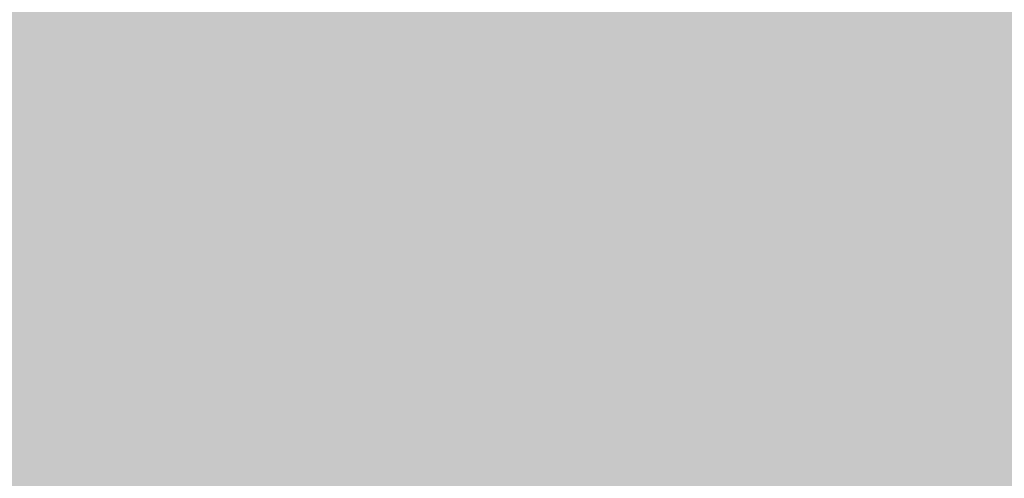
# Model space of a CAD drawing. Units: millimetres. Extents: x 0 to 2267, y 0 to 1823.
# Tile 146 of 256: x 1823.16 to 1833.61, y 1122.41 to 1127.28. Entities that reach past the tile are written whole.
import ezdxf

# ---------------------------------------------------------------- set-up
doc = ezdxf.new("R2010")
doc.units = ezdxf.units.MM
doc.header["$MEASUREMENT"] = 0
doc.layers.add('M-DIMS', color=2, linetype='Continuous', lineweight=25)
doc.layers.add('M-HATC', color=252, linetype='Continuous', lineweight=18)
doc.styles.get("Standard").update_dxf_attribs({"font": 'arial.ttf'})
doc.dimstyles.get("Standard").update_dxf_attribs({"dimtxt": 7, "dimasz": 4, "dimexe": 0.18, "dimexo": 0.0625, "dimgap": 0.09, "dimtad": 0, "dimdec": 0, "dimzin": 0, "dimdsep": 46, "dimtxsty": 'Standard', "dimcen": 0.09, "dimadec": 0, "dimazin": 0, "dimtfac": 1, "dimtdec": 0, "dimtofl": 0, "dimtmove": 0, "dimatfit": 3, "dimfxl": 1, "dimtolj": 1, "dimtzin": 0, "dimarcsym": 0})

# ---------------------------------------------------------------- blocks, each defined once
blk = doc.blocks.new('*D1')
at = {"layer": 'Defpoints', "color": 0, "transparency": 16777216}
for p in [(1593.429, 1127.417), (1843.429, 1127.417), (1843.429, 955.628)]:
    blk.add_point(p, dxfattribs=at)
at = {"layer": 'M-DIMS', "color": 0, "lineweight": -2, "transparency": 16777216}
for p, q in [((1593.429, 1127.355), (1593.429, 955.448)), ((1843.429, 1127.355), (1843.429, 955.448)), ((1597.429, 955.628), (1710.558, 955.628)), ((1839.429, 955.628), (1726.3, 955.628))]:
    blk.add_line(p, q, dxfattribs=at)
at = {"layer": 'M-DIMS', "color": 0, "transparency": 16777216}
for points in [[(1597.429, 956.294), (1597.429, 954.961), (1593.429, 955.628)], [(1839.429, 956.294), (1839.429, 954.961), (1843.429, 955.628)]]:
    blk.add_solid(points, dxfattribs=at)
at = {"layer": 'M-DIMS', "color": 0, "transparency": 16777216, "insert": (1718.429, 955.628), "char_height": 7, "attachment_point": 5}
blk.add_mtext('\\A1;250', dxfattribs=at)

msp = doc.modelspace()

# ---------------------------------------------------------------- hatches: boundary and pattern name
at = {"layer": 'M-HATC'}
h = msp.add_hatch(color=256, dxfattribs=at)
h.dxf.hatch_style = 1
h.paths.add_polyline_path([(2055.771, 1603.062), (1381.087, 1603.062), (1381.087, 1598.062), (2055.771, 1598.062)])
h.paths.add_polyline_path([(2055.771, 1598.062), (1381.087, 1598.062), (1381.087, 1593.062), (2055.771, 1593.062)])
h.paths.add_polyline_path([(2051.307, 1536.761), (1385.55, 1536.761), (1385.55, 1526.761), (1387.55, 1526.761), (1388.537, 1525.053), (1385.332, 1521.233), (1385.332, 1521.223), (2050.254, 1522.749), (2048.321, 1525.053), (2049.307, 1526.761), (2051.307, 1526.761)])
edge = h.paths.add_edge_path()
edge.add_arc((1847.535, 1379.149), 135, 222.60306, 222.89085, ccw=False)
edge.add_line((1748.166, 1287.766), (1683.092, 1287.766))
edge.add_arc((1583.724, 1379.149), 135, 317.10915, 317.39694, ccw=False)
edge.add_arc((1678.969, 1290.671), 5, 222.8909, 317.1091, ccw=False)
edge.add_arc((1774.213, 1379.149), 135, 222.60306, 222.89085, ccw=False)
edge.add_line((1674.845, 1287.766), (1609.771, 1287.766))
edge.add_arc((1510.403, 1379.149), 135, 317.10915, 317.39694, ccw=False)
edge.add_arc((1605.647, 1290.671), 5, 222.8909, 317.1091, ccw=False)
edge.add_arc((1700.892, 1379.149), 135, 222.60306, 222.89085, ccw=False)
edge.add_line((1601.524, 1287.766), (1536.45, 1287.766))
edge.add_arc((1437.081, 1379.149), 135, 317.10915, 317.39694, ccw=False)
edge.add_arc((1532.326, 1290.671), 5, 222.8909, 317.1091, ccw=False)
edge.add_arc((1627.571, 1379.149), 135, 222.60306, 222.89085, ccw=False)
edge.add_line((1528.203, 1287.766), (1505.929, 1287.766))
edge.add_spline(control_points=[(1505.929, 1287.766), (1504.262, 1287.766), (1504.262, 1282.766), (1505.929, 1282.766)], knot_values=[0, 0, 0, 0, 5, 5, 5, 5], degree=3, periodic=0)
edge.add_line((1505.929, 1282.766), (1930.929, 1282.766))
edge.add_spline(control_points=[(1930.929, 1282.766), (1932.596, 1282.766), (1932.596, 1287.766), (1930.929, 1287.766)], knot_values=[0, 0, 0, 0, 5, 5, 5, 5], degree=3, periodic=0)
edge.add_line((1930.929, 1287.766), (1903.056, 1287.766))
edge.add_arc((1803.688, 1379.149), 135, 317.10915, 317.39694, ccw=False)
edge.add_arc((1898.932, 1290.671), 5, 222.8909, 317.1091, ccw=False)
edge.add_arc((1994.177, 1379.149), 135, 222.60306, 222.89085, ccw=False)
edge.add_line((1894.809, 1287.766), (1829.735, 1287.766))
edge.add_arc((1730.366, 1379.149), 135, 317.10915, 317.39694, ccw=False)
edge.add_arc((1825.611, 1290.671), 5, 222.8909, 317.1091, ccw=False)
edge.add_arc((1920.856, 1379.149), 135, 222.60306, 222.89085, ccw=False)
edge.add_line((1821.487, 1287.766), (1756.413, 1287.766))
edge.add_arc((1657.045, 1379.149), 135, 317.10915, 317.39694, ccw=False)
edge.add_arc((1752.29, 1290.671), 5, 222.8909, 317.1091, ccw=False)
edge = h.paths.add_edge_path()
edge.add_spline(control_points=[(1843.429, 1227.247), (1845.096, 1227.247), (1845.096, 1232.247), (1843.429, 1232.247)], knot_values=[0, 0, 0, 0, 5, 5, 5, 5], degree=3, periodic=0)
edge.add_line((1843.429, 1232.247), (1593.429, 1232.247))
edge.add_spline(control_points=[(1593.429, 1232.247), (1591.762, 1232.247), (1591.762, 1227.247), (1593.429, 1227.247)], knot_values=[0, 0, 0, 0, 5, 5, 5, 5], degree=3, periodic=0)
edge.add_line((1593.429, 1227.247), (1843.429, 1227.247))
h.paths.add_polyline_path([(1905.929, 1127.417), (1530.929, 1127.417, 0.414214), (1520.929, 1117.417), (1530.929, 1117.417), (1915.929, 1117.417, 0.414214)])
edge = h.paths.add_edge_path()
edge.add_arc((1397.086, 1498.408), 12.73, 90.7821, 190.8787, ccw=False)
edge.add_line((1396.912, 1511.136), (1428.01, 1511.349))
edge.add_line((1428.01, 1511.349), (1433.01, 1511.349))
edge.add_line((1433.01, 1511.349), (1434.439, 1511.349))
edge.add_arc((1419.474, 1498.08), 20, 41.561, 74.0821)
edge.add_line((1424.959, 1517.314), (1399.935, 1517.256))
edge.add_spline(control_points=[(1399.931, 1517.256), (1399.884, 1517.213), (1399.833, 1517.169), (1399.777, 1517.124)], knot_values=[11.567499, 11.567499, 11.567499, 11.567499, 11.814249, 11.814249, 11.814249, 11.814249], degree=3, periodic=0)
edge.add_spline(control_points=[(1399.633, 1517.01), (1399.583, 1516.972), (1399.531, 1516.934), (1399.476, 1516.895)], knot_values=[11.167718, 11.167718, 11.167718, 11.167718, 11.365188, 11.365188, 11.365188, 11.365188], degree=3, periodic=0)
edge.add_spline(control_points=[(1399.34, 1516.8), (1399.151, 1516.672), (1398.938, 1516.538), (1398.704, 1516.399)], knot_values=[10.376405, 10.376405, 10.376405, 10.376405, 11.00994, 11.00994, 11.00994, 11.00994], degree=3, periodic=0)
edge.add_spline(control_points=[(1398.657, 1516.372), (1398.579, 1516.326), (1398.498, 1516.28), (1398.415, 1516.233)], knot_values=[10.125175, 10.125175, 10.125175, 10.125175, 10.334406, 10.334406, 10.334406, 10.334406], degree=3, periodic=0)
edge.add_spline(control_points=[(1398.264, 1516.149), (1398.196, 1516.111), (1398.126, 1516.073), (1398.055, 1516.035)], knot_values=[9.832246, 9.832246, 9.832246, 9.832246, 9.999658, 9.999658, 9.999658, 9.999658], degree=3, periodic=0)
edge.add_spline(control_points=[(1397.999, 1516.005), (1397.731, 1515.862), (1397.446, 1515.717), (1397.147, 1515.571)], knot_values=[9.161808, 9.161808, 9.161808, 9.161808, 9.787769, 9.787769, 9.787769, 9.787769], degree=3, periodic=0)
edge.add_spline(control_points=[(1397.147, 1515.571), (1396.842, 1515.423), (1396.522, 1515.274), (1396.191, 1515.126)], knot_values=[8.524455, 8.524455, 8.524455, 8.524455, 9.161808, 9.161808, 9.161808, 9.161808], degree=3, periodic=0)
edge.add_spline(control_points=[(1396.078, 1515.076), (1395.985, 1515.035), (1395.892, 1514.994), (1395.798, 1514.953)], knot_values=[8.275193, 8.275193, 8.275193, 8.275193, 8.451726, 8.451726, 8.451726, 8.451726], degree=3, periodic=0)
edge.add_spline(control_points=[(1395.602, 1514.869), (1395.5, 1514.826), (1395.397, 1514.782), (1395.293, 1514.739)], knot_values=[7.962917, 7.962917, 7.962917, 7.962917, 8.152764, 8.152764, 8.152764, 8.152764], degree=3, periodic=0)
edge.add_spline(control_points=[(1395.212, 1514.706), (1394.828, 1514.547), (1394.435, 1514.393), (1394.036, 1514.244)], knot_values=[7.21254, 7.21254, 7.21254, 7.21254, 7.913148, 7.913148, 7.913148, 7.913148], degree=3, periodic=0)
edge.add_spline(control_points=[(1394.036, 1514.244), (1393.708, 1514.121), (1393.375, 1514.003), (1393.043, 1513.889)], knot_values=[6.633733, 6.633733, 6.633733, 6.633733, 7.21254, 7.21254, 7.21254, 7.21254], degree=3, periodic=0)
edge.add_spline(control_points=[(1392.821, 1513.815), (1392.72, 1513.781), (1392.618, 1513.748), (1392.517, 1513.715)], knot_values=[6.328796, 6.328796, 6.328796, 6.328796, 6.505493, 6.505493, 6.505493, 6.505493], degree=3, periodic=0)
edge.add_spline(control_points=[(1392.517, 1513.715), (1392.319, 1513.652), (1392.121, 1513.59), (1391.924, 1513.531)], knot_values=[5.984605, 5.984605, 5.984605, 5.984605, 6.328796, 6.328796, 6.328796, 6.328796], degree=3, periodic=0)
edge.add_spline(control_points=[(1391.792, 1513.491), (1391.312, 1513.35), (1390.838, 1513.224), (1390.378, 1513.117)], knot_values=[5.066697, 5.066697, 5.066697, 5.066697, 5.907055, 5.907055, 5.907055, 5.907055], degree=3, periodic=0)
edge.add_spline(control_points=[(1390.378, 1513.117), (1390.18, 1513.071), (1389.984, 1513.028), (1389.791, 1512.99)], knot_values=[4.70367, 4.70367, 4.70367, 4.70367, 5.066695, 5.066695, 5.066695, 5.066695], degree=3, periodic=0)
edge.add_spline(control_points=[(1389.422, 1512.92), (1389.246, 1512.889), (1389.073, 1512.862), (1388.904, 1512.838)], knot_values=[4.130571, 4.130571, 4.130571, 4.130571, 4.469816, 4.469816, 4.469816, 4.469816], degree=3, periodic=0)
edge.add_spline(control_points=[(1388.904, 1512.838), (1388.591, 1512.795), (1388.291, 1512.764), (1388.007, 1512.749)], knot_values=[3.504031, 3.504031, 3.504031, 3.504031, 4.130571, 4.130571, 4.130571, 4.130571], degree=3, periodic=0)
edge.add_spline(control_points=[(1387.936, 1512.746), (1387.854, 1512.742), (1387.773, 1512.74), (1387.694, 1512.739)], knot_values=[3.268866, 3.268866, 3.268866, 3.268866, 3.451164, 3.451164, 3.451164, 3.451164], degree=3, periodic=0)
edge.add_spline(control_points=[(1387.335, 1512.744), (1387.208, 1512.75), (1387.085, 1512.76), (1386.967, 1512.774)], knot_values=[2.670686, 2.670686, 2.670686, 2.670686, 2.984, 2.984, 2.984, 2.984], degree=3, periodic=0)
edge.add_spline(control_points=[(1386.833, 1512.792), (1386.821, 1512.794), (1386.809, 1512.796), (1386.797, 1512.798)], knot_values=[2.516981, 2.516981, 2.516981, 2.516981, 2.549528, 2.549528, 2.549528, 2.549528], degree=3, periodic=0)
edge.add_spline(control_points=[(1386.453, 1512.873), (1386.426, 1512.881), (1386.399, 1512.889), (1386.373, 1512.897)], knot_values=[2.095869, 2.095869, 2.095869, 2.095869, 2.17941, 2.17941, 2.17941, 2.17941], degree=3, periodic=0)
edge.add_spline(control_points=[(1386.069, 1513.019), (1386.063, 1513.022), (1386.058, 1513.025), (1386.052, 1513.028)], knot_values=[1.72453, 1.72453, 1.72453, 1.72453, 1.745933, 1.745933, 1.745933, 1.745933], degree=3, periodic=0)
edge.add_arc((1399.474, 1498.08), 20, 131.8243, 180)
edge.add_arc((1630.334, 1505.548), 250.971, 181.70518, 236.42798)
edge.add_arc((1605.34, 1483.304), 218.782, 238.66083, 243.34961)
edge.add_arc((1647.091, 1510.359), 262.899, 183.12984, 237.85344, ccw=False)
h.paths.add_polyline_path([(1406.537, 1391.964, 0.149382), (1491.551, 1296.442, -0.129517)], flags=17)
edge = h.paths.add_edge_path()
edge.add_arc((2037.384, 1498.08), 20, 0, 48.2659)
edge.add_spline(control_points=[(2050.697, 1513.005), (2050.651, 1512.985), (2050.603, 1512.966), (2050.554, 1512.948)], knot_values=[1.835652, 1.835652, 1.835652, 1.835652, 2.000781, 2.000781, 2.000781, 2.000781], degree=3, periodic=0)
edge.add_spline(control_points=[(2050.462, 1512.917), (2050.479, 1512.922), (2050.496, 1512.928), (2050.513, 1512.934)], knot_values=[2.045477, 2.045477, 2.045477, 2.045477, 2.101389, 2.101389, 2.101389, 2.101389], degree=3, periodic=0)
edge.add_spline(control_points=[(2050.129, 1512.834), (2050.198, 1512.847), (2050.266, 1512.862), (2050.331, 1512.879)], knot_values=[2.237629, 2.237629, 2.237629, 2.237629, 2.435841, 2.435841, 2.435841, 2.435841], degree=3, periodic=0)
edge.add_spline(control_points=[(2050.095, 1512.828), (2050.106, 1512.83), (2050.118, 1512.832), (2050.129, 1512.834)], knot_values=[2.435841, 2.435841, 2.435841, 2.435841, 2.468321, 2.468321, 2.468321, 2.468321], degree=3, periodic=0)
edge.add_spline(control_points=[(2049.784, 1512.785), (2049.855, 1512.792), (2049.924, 1512.801), (2049.992, 1512.811)], knot_values=[2.563852, 2.563852, 2.563852, 2.563852, 2.748541, 2.748541, 2.748541, 2.748541], degree=3, periodic=0)
edge.add_spline(control_points=[(2049.405, 1512.762), (2049.536, 1512.765), (2049.663, 1512.773), (2049.784, 1512.785)], knot_values=[2.748541, 2.748541, 2.748541, 2.748541, 3.064882, 3.064882, 3.064882, 3.064882], degree=3, periodic=0)
edge.add_spline(control_points=[(2049.17, 1512.76), (2049.234, 1512.759), (2049.297, 1512.759), (2049.358, 1512.761)], knot_values=[3.102309, 3.102309, 3.102309, 3.102309, 3.2503, 3.2503, 3.2503, 3.2503], degree=3, periodic=0)
edge.add_spline(control_points=[(2048.857, 1512.769), (2048.964, 1512.764), (2049.068, 1512.761), (2049.17, 1512.76)], knot_values=[3.2503, 3.2503, 3.2503, 3.2503, 3.486069, 3.486069, 3.486069, 3.486069], degree=3, periodic=0)
edge.add_spline(control_points=[(2048.692, 1512.779), (2048.373, 1512.801), (2048.035, 1512.841), (2047.682, 1512.897)], knot_values=[3.606429, 3.606429, 3.606429, 3.606429, 4.2989, 4.2989, 4.2989, 4.2989], degree=3, periodic=0)
edge.add_spline(control_points=[(2047.682, 1512.897), (2047.546, 1512.919), (2047.408, 1512.942), (2047.268, 1512.969)], knot_values=[4.2989, 4.2989, 4.2989, 4.2989, 4.565769, 4.565769, 4.565769, 4.565769], degree=3, periodic=0)
edge.add_spline(control_points=[(2047.268, 1512.969), (2047.145, 1512.991), (2047.021, 1513.016), (2046.895, 1513.042)], knot_values=[4.565769, 4.565769, 4.565769, 4.565769, 4.799971, 4.799971, 4.799971, 4.799971], degree=3, periodic=0)
edge.add_spline(control_points=[(2046.895, 1513.042), (2046.529, 1513.119), (2046.151, 1513.209), (2045.768, 1513.311)], knot_values=[4.799971, 4.799971, 4.799971, 4.799971, 5.483718, 5.483718, 5.483718, 5.483718], degree=3, periodic=0)
edge.add_spline(control_points=[(2045.768, 1513.311), (2045.372, 1513.415), (2044.97, 1513.532), (2044.566, 1513.659)], knot_values=[5.483718, 5.483718, 5.483718, 5.483718, 6.187866, 6.187866, 6.187866, 6.187866], degree=3, periodic=0)
edge.add_spline(control_points=[(2044.566, 1513.659), (2044.415, 1513.706), (2044.263, 1513.755), (2044.112, 1513.805)], knot_values=[6.187866, 6.187866, 6.187866, 6.187866, 6.451551, 6.451551, 6.451551, 6.451551], degree=3, periodic=0)
edge.add_spline(control_points=[(2044.112, 1513.805), (2043.997, 1513.843), (2043.882, 1513.881), (2043.767, 1513.92)], knot_values=[6.451551, 6.451551, 6.451551, 6.451551, 6.651434, 6.651434, 6.651434, 6.651434], degree=3, periodic=0)
edge.add_spline(control_points=[(2043.767, 1513.92), (2043.372, 1514.055), (2042.977, 1514.198), (2042.589, 1514.346)], knot_values=[6.651434, 6.651434, 6.651434, 6.651434, 7.338879, 7.338879, 7.338879, 7.338879], degree=3, periodic=0)
edge.add_spline(control_points=[(2042.589, 1514.346), (2042.164, 1514.507), (2041.746, 1514.675), (2041.341, 1514.846)], knot_values=[7.338879, 7.338879, 7.338879, 7.338879, 8.089209, 8.089209, 8.089209, 8.089209], degree=3, periodic=0)
edge.add_spline(control_points=[(2041.341, 1514.846), (2041.103, 1514.946), (2040.869, 1515.048), (2040.64, 1515.15)], knot_values=[8.089209, 8.089209, 8.089209, 8.089209, 8.529587, 8.529587, 8.529587, 8.529587], degree=3, periodic=0)
edge.add_spline(control_points=[(2040.51, 1515.209), (2040.082, 1515.402), (2039.675, 1515.597), (2039.295, 1515.789)], knot_values=[8.613818, 8.613818, 8.613818, 8.613818, 9.44571, 9.44571, 9.44571, 9.44571], degree=3, periodic=0)
edge.add_spline(control_points=[(2039.295, 1515.789), (2039.062, 1515.907), (2038.839, 1516.025), (2038.629, 1516.14)], knot_values=[9.44571, 9.44571, 9.44571, 9.44571, 9.956404, 9.956404, 9.956404, 9.956404], degree=3, periodic=0)
edge.add_spline(control_points=[(2038.629, 1516.14), (2038.519, 1516.2), (2038.412, 1516.26), (2038.309, 1516.319)], knot_values=[9.956404, 9.956404, 9.956404, 9.956404, 10.223542, 10.223542, 10.223542, 10.223542], degree=3, periodic=0)
edge.add_spline(control_points=[(2038.309, 1516.319), (2038.214, 1516.374), (2038.122, 1516.428), (2038.033, 1516.481)], knot_values=[10.223542, 10.223542, 10.223542, 10.223542, 10.47051, 10.47051, 10.47051, 10.47051], degree=3, periodic=0)
edge.add_spline(control_points=[(2038.033, 1516.481), (2037.786, 1516.63), (2037.564, 1516.773), (2037.372, 1516.909)], knot_values=[10.47051, 10.47051, 10.47051, 10.47051, 11.15767, 11.15767, 11.15767, 11.15767], degree=3, periodic=0)
edge.add_spline(control_points=[(2037.372, 1516.909), (2037.279, 1516.975), (2037.193, 1517.04), (2037.114, 1517.102)], knot_values=[11.15767, 11.15767, 11.15767, 11.15767, 11.49227, 11.49227, 11.49227, 11.49227], degree=3, periodic=0)
edge.add_spline(control_points=[(2036.856, 1517.326), (2036.915, 1517.269), (2036.981, 1517.21), (2037.056, 1517.149)], knot_values=[11.577341, 11.577341, 11.577341, 11.577341, 11.91035, 11.91035, 11.91035, 11.91035], degree=3, periodic=0)
edge.add_spline(control_points=[(2036.807, 1517.375), (2036.823, 1517.359), (2036.839, 1517.342), (2036.856, 1517.326)], knot_values=[11.91035, 11.91035, 11.91035, 11.91035, 12.007402, 12.007402, 12.007402, 12.007402], degree=3, periodic=0)
edge.add_spline(control_points=[(2036.702, 1517.494), (2036.71, 1517.483), (2036.72, 1517.472), (2036.729, 1517.461)], knot_values=[12.184155, 12.184155, 12.184155, 12.184155, 12.255409, 12.255409, 12.255409, 12.255409], degree=3, periodic=0)
edge.add_spline(control_points=[(2036.616, 1517.621), (2036.62, 1517.613), (2036.624, 1517.606), (2036.629, 1517.598)], knot_values=[12.487913, 12.487913, 12.487913, 12.487913, 12.541035, 12.541035, 12.541035, 12.541035], degree=3, periodic=0)
edge.add_spline(control_points=[(2036.563, 1517.786), (2036.564, 1517.779), (2036.564, 1517.773), (2036.565, 1517.766)], knot_values=[12.911761, 12.911761, 12.911761, 12.911761, 12.968286, 12.968286, 12.968286, 12.968286], degree=3, periodic=0)
edge.add_spline(control_points=[(2036.617, 1517.93), (2036.612, 1517.926), (2036.609, 1517.921), (2036.605, 1517.916)], knot_values=[13.382527, 13.382527, 13.382527, 13.382527, 13.433791, 13.433791, 13.433791, 13.433791], degree=3, periodic=0)
edge.add_spline(control_points=[(2036.749, 1518.017), (2036.736, 1518.012), (2036.724, 1518.006), (2036.712, 1518)], knot_values=[13.726299, 13.726299, 13.726299, 13.726299, 13.809928, 13.809928, 13.809928, 13.809928], degree=3, periodic=0)
edge.add_spline(control_points=[(2036.86, 1518.053), (2036.839, 1518.047), (2036.818, 1518.042), (2036.799, 1518.035)], knot_values=[13.910887, 13.910887, 13.910887, 13.910887, 14.02153, 14.02153, 14.02153, 14.02153], degree=3, periodic=0)
edge.add_line((2036.964, 1518.08), (2032.384, 1518.08))
edge.add_line((2032.384, 1518.08), (2027.384, 1518.08))
edge.add_line((2027.384, 1518.08), (2022.384, 1518.08))
edge.add_line((2022.384, 1518.08), (2017.384, 1518.08))
edge.add_arc((2017.384, 1498.08), 20, 90, 138.439)
edge.add_line((2002.419, 1511.349), (2003.848, 1511.349))
edge.add_line((2003.848, 1511.349), (2008.848, 1511.349))
edge.add_line((2008.848, 1511.349), (2039.772, 1511.138))
edge.add_arc((2039.772, 1498.408), 12.73, -10.8787, 90, ccw=False)
edge.add_arc((1789.767, 1510.359), 262.899, 302.14656, 356.87016, ccw=False)
edge.add_arc((1831.518, 1483.304), 218.782, 296.65039, 301.33917)
edge.add_arc((1806.524, 1505.548), 250.971, 303.57202, 358.29482)
h.paths.add_polyline_path([(2030.321, 1391.964, -0.129517), (1945.307, 1296.442, 0.149382)], flags=17)
edge = h.paths.add_edge_path()
edge.add_spline(control_points=[(2037.246, 1518.082), (2037.29, 1518.081), (2037.336, 1518.08), (2037.384, 1518.08)], knot_values=[0.000012, 0.000012, 0.000012, 0.000012, 0.144754, 0.144754, 0.144754, 0.144754], degree=3, periodic=0)
edge.add_line((2037.336, 1518.08), (2037.01, 1518.08))
edge.add_spline(control_points=[(2037.01, 1518.08), (2036.982, 1518.077), (2036.956, 1518.073), (2036.931, 1518.068)], knot_values=[14.13465, 14.13465, 14.13465, 14.13465, 14.247197, 14.247197, 14.247197, 14.247197], degree=3, periodic=0)
edge.add_spline(control_points=[(2036.931, 1518.068), (2036.928, 1518.067), (2036.924, 1518.067), (2036.921, 1518.066)], knot_values=[14.118315, 14.118315, 14.118315, 14.118315, 14.13465, 14.13465, 14.13465, 14.13465], degree=3, periodic=0)
edge.add_spline(control_points=[(2036.921, 1518.066), (2036.912, 1518.064), (2036.903, 1518.063), (2036.895, 1518.061)], knot_values=[14.078086, 14.078086, 14.078086, 14.078086, 14.118315, 14.118315, 14.118315, 14.118315], degree=3, periodic=0)
edge.add_spline(control_points=[(2036.895, 1518.061), (2036.883, 1518.058), (2036.872, 1518.056), (2036.86, 1518.053)], knot_values=[14.02153, 14.02153, 14.02153, 14.02153, 14.078086, 14.078086, 14.078086, 14.078086], degree=3, periodic=0)
edge.add_spline(control_points=[(2036.86, 1518.053), (2036.839, 1518.047), (2036.818, 1518.042), (2036.799, 1518.035)], knot_values=[13.910887, 13.910887, 13.910887, 13.910887, 14.02153, 14.02153, 14.02153, 14.02153], degree=3, periodic=0)
edge.add_spline(control_points=[(2036.799, 1518.035), (2036.798, 1518.035), (2036.797, 1518.035), (2036.797, 1518.035)], knot_values=[13.906906, 13.906906, 13.906906, 13.906906, 13.910887, 13.910887, 13.910887, 13.910887], degree=3, periodic=0)
edge.add_spline(control_points=[(2036.797, 1518.035), (2036.788, 1518.032), (2036.78, 1518.029), (2036.772, 1518.026)], knot_values=[13.857826, 13.857826, 13.857826, 13.857826, 13.906906, 13.906906, 13.906906, 13.906906], degree=3, periodic=0)
edge.add_spline(control_points=[(2036.772, 1518.026), (2036.764, 1518.023), (2036.756, 1518.02), (2036.749, 1518.017)], knot_values=[13.809928, 13.809928, 13.809928, 13.809928, 13.857826, 13.857826, 13.857826, 13.857826], degree=3, periodic=0)
edge.add_spline(control_points=[(2036.749, 1518.017), (2036.736, 1518.012), (2036.724, 1518.006), (2036.712, 1518)], knot_values=[13.726299, 13.726299, 13.726299, 13.726299, 13.809928, 13.809928, 13.809928, 13.809928], degree=3, periodic=0)
edge.add_spline(control_points=[(2036.712, 1518), (2036.712, 1518), (2036.712, 1518), (2036.711, 1518)], knot_values=[13.723993, 13.723993, 13.723993, 13.723993, 13.726299, 13.726299, 13.726299, 13.726299], degree=3, periodic=0)
edge.add_spline(control_points=[(2036.711, 1518), (2036.706, 1517.997), (2036.701, 1517.994), (2036.696, 1517.992)], knot_values=[13.686536, 13.686536, 13.686536, 13.686536, 13.723993, 13.723993, 13.723993, 13.723993], degree=3, periodic=0)
edge.add_spline(control_points=[(2036.696, 1517.992), (2036.692, 1517.989), (2036.687, 1517.987), (2036.683, 1517.984)], knot_values=[13.651251, 13.651251, 13.651251, 13.651251, 13.686536, 13.686536, 13.686536, 13.686536], degree=3, periodic=0)
edge.add_spline(control_points=[(2036.683, 1517.984), (2036.676, 1517.98), (2036.67, 1517.976), (2036.664, 1517.971)], knot_values=[13.596804, 13.596804, 13.596804, 13.596804, 13.651251, 13.651251, 13.651251, 13.651251], degree=3, periodic=0)
edge.add_spline(control_points=[(2036.664, 1517.971), (2036.664, 1517.971), (2036.663, 1517.971), (2036.663, 1517.971)], knot_values=[13.593956, 13.593956, 13.593956, 13.593956, 13.596804, 13.596804, 13.596804, 13.596804], degree=3, periodic=0)
edge.add_spline(control_points=[(2036.663, 1517.971), (2036.66, 1517.969), (2036.658, 1517.967), (2036.655, 1517.965)], knot_values=[13.570322, 13.570322, 13.570322, 13.570322, 13.593956, 13.593956, 13.593956, 13.593956], degree=3, periodic=0)
edge.add_spline(control_points=[(2036.655, 1517.965), (2036.653, 1517.963), (2036.65, 1517.961), (2036.647, 1517.959)], knot_values=[13.545477, 13.545477, 13.545477, 13.545477, 13.570322, 13.570322, 13.570322, 13.570322], degree=3, periodic=0)
edge.add_spline(control_points=[(2036.647, 1517.959), (2036.647, 1517.959), (2036.647, 1517.959), (2036.647, 1517.959)], knot_values=[13.543931, 13.543931, 13.543931, 13.543931, 13.545477, 13.545477, 13.545477, 13.545477], degree=3, periodic=0)
edge.add_spline(control_points=[(2036.647, 1517.959), (2036.641, 1517.954), (2036.636, 1517.949), (2036.631, 1517.945)], knot_values=[13.488237, 13.488237, 13.488237, 13.488237, 13.543931, 13.543931, 13.543931, 13.543931], degree=3, periodic=0)
edge.add_spline(control_points=[(2036.631, 1517.945), (2036.628, 1517.942), (2036.626, 1517.94), (2036.623, 1517.937)], knot_values=[13.460307, 13.460307, 13.460307, 13.460307, 13.488237, 13.488237, 13.488237, 13.488237], degree=3, periodic=0)
edge.add_spline(control_points=[(2036.623, 1517.937), (2036.622, 1517.936), (2036.62, 1517.934), (2036.618, 1517.932)], knot_values=[13.439712, 13.439712, 13.439712, 13.439712, 13.460307, 13.460307, 13.460307, 13.460307], degree=3, periodic=0)
edge.add_spline(control_points=[(2036.618, 1517.932), (2036.618, 1517.931), (2036.617, 1517.931), (2036.617, 1517.93)], knot_values=[13.433791, 13.433791, 13.433791, 13.433791, 13.439712, 13.439712, 13.439712, 13.439712], degree=3, periodic=0)
edge.add_spline(control_points=[(2036.617, 1517.93), (2036.612, 1517.926), (2036.609, 1517.921), (2036.605, 1517.916)], knot_values=[13.382527, 13.382527, 13.382527, 13.382527, 13.433791, 13.433791, 13.433791, 13.433791], degree=3, periodic=0)
edge.add_spline(control_points=[(2036.605, 1517.916), (2036.603, 1517.913), (2036.6, 1517.91), (2036.598, 1517.907)], knot_values=[13.350017, 13.350017, 13.350017, 13.350017, 13.382527, 13.382527, 13.382527, 13.382527], degree=3, periodic=0)
edge.add_spline(control_points=[(2036.598, 1517.907), (2036.597, 1517.906), (2036.596, 1517.904), (2036.595, 1517.903)], knot_values=[13.333922, 13.333922, 13.333922, 13.333922, 13.350017, 13.350017, 13.350017, 13.350017], degree=3, periodic=0)
edge.add_spline(control_points=[(2036.595, 1517.903), (2036.595, 1517.902), (2036.594, 1517.901), (2036.593, 1517.9)], knot_values=[13.323828, 13.323828, 13.323828, 13.323828, 13.333922, 13.333922, 13.333922, 13.333922], degree=3, periodic=0)
edge.add_spline(control_points=[(2036.593, 1517.9), (2036.59, 1517.895), (2036.588, 1517.891), (2036.585, 1517.886)], knot_values=[13.277545, 13.277545, 13.277545, 13.277545, 13.323828, 13.323828, 13.323828, 13.323828], degree=3, periodic=0)
edge.add_spline(control_points=[(2036.585, 1517.886), (2036.584, 1517.883), (2036.582, 1517.879), (2036.58, 1517.875)], knot_values=[13.240119, 13.240119, 13.240119, 13.240119, 13.277545, 13.277545, 13.277545, 13.277545], degree=3, periodic=0)
edge.add_spline(control_points=[(2036.58, 1517.875), (2036.58, 1517.874), (2036.579, 1517.873), (2036.578, 1517.872)], knot_values=[13.228211, 13.228211, 13.228211, 13.228211, 13.240119, 13.240119, 13.240119, 13.240119], degree=3, periodic=0)
edge.add_spline(control_points=[(2036.578, 1517.872), (2036.578, 1517.87), (2036.577, 1517.869), (2036.577, 1517.868)], knot_values=[13.215717, 13.215717, 13.215717, 13.215717, 13.228211, 13.228211, 13.228211, 13.228211], degree=3, periodic=0)
edge.add_spline(control_points=[(2036.577, 1517.868), (2036.575, 1517.864), (2036.574, 1517.86), (2036.573, 1517.857)], knot_values=[13.179847, 13.179847, 13.179847, 13.179847, 13.215717, 13.215717, 13.215717, 13.215717], degree=3, periodic=0)
edge.add_spline(control_points=[(2036.573, 1517.857), (2036.571, 1517.851), (2036.57, 1517.846), (2036.569, 1517.841)], knot_values=[13.132017, 13.132017, 13.132017, 13.132017, 13.179847, 13.179847, 13.179847, 13.179847], degree=3, periodic=0)
edge.add_spline(control_points=[(2036.569, 1517.841), (2036.568, 1517.84), (2036.568, 1517.839), (2036.568, 1517.838)], knot_values=[13.122482, 13.122482, 13.122482, 13.122482, 13.132017, 13.132017, 13.132017, 13.132017], degree=3, periodic=0)
edge.add_spline(control_points=[(2036.568, 1517.838), (2036.568, 1517.836), (2036.567, 1517.835), (2036.567, 1517.833)], knot_values=[13.105592, 13.105592, 13.105592, 13.105592, 13.122482, 13.122482, 13.122482, 13.122482], degree=3, periodic=0)
edge.add_spline(control_points=[(2036.567, 1517.833), (2036.566, 1517.829), (2036.566, 1517.826), (2036.565, 1517.822)], knot_values=[13.074063, 13.074063, 13.074063, 13.074063, 13.105592, 13.105592, 13.105592, 13.105592], degree=3, periodic=0)
edge.add_spline(control_points=[(2036.565, 1517.822), (2036.565, 1517.822), (2036.565, 1517.822), (2036.565, 1517.822)], knot_values=[13.074043, 13.074043, 13.074043, 13.074043, 13.074063, 13.074063, 13.074063, 13.074063], degree=3, periodic=0)
edge.add_spline(control_points=[(2036.565, 1517.822), (2036.564, 1517.816), (2036.564, 1517.811), (2036.564, 1517.805)], knot_values=[13.021884, 13.021884, 13.021884, 13.021884, 13.074043, 13.074043, 13.074043, 13.074043], degree=3, periodic=0)
edge.add_spline(control_points=[(2036.564, 1517.805), (2036.564, 1517.804), (2036.564, 1517.803), (2036.564, 1517.803)], knot_values=[13.01674, 13.01674, 13.01674, 13.01674, 13.021884, 13.021884, 13.021884, 13.021884], degree=3, periodic=0)
edge.add_spline(control_points=[(2036.564, 1517.803), (2036.563, 1517.801), (2036.563, 1517.798), (2036.563, 1517.796)], knot_values=[12.996438, 12.996438, 12.996438, 12.996438, 13.01674, 13.01674, 13.01674, 13.01674], degree=3, periodic=0)
edge.add_spline(control_points=[(2036.563, 1517.796), (2036.563, 1517.793), (2036.563, 1517.789), (2036.563, 1517.786)], knot_values=[12.968286, 12.968286, 12.968286, 12.968286, 12.996438, 12.996438, 12.996438, 12.996438], degree=3, periodic=0)
edge.add_spline(control_points=[(2036.563, 1517.786), (2036.564, 1517.779), (2036.564, 1517.773), (2036.565, 1517.766)], knot_values=[12.911761, 12.911761, 12.911761, 12.911761, 12.968286, 12.968286, 12.968286, 12.968286], degree=3, periodic=0)
edge.add_spline(control_points=[(2036.565, 1517.766), (2036.565, 1517.766), (2036.565, 1517.766), (2036.565, 1517.766)], knot_values=[12.911017, 12.911017, 12.911017, 12.911017, 12.911761, 12.911761, 12.911761, 12.911761], degree=3, periodic=0)
edge.add_spline(control_points=[(2036.565, 1517.766), (2036.565, 1517.762), (2036.566, 1517.759), (2036.566, 1517.756)], knot_values=[12.88528, 12.88528, 12.88528, 12.88528, 12.911017, 12.911017, 12.911017, 12.911017], degree=3, periodic=0)
edge.add_spline(control_points=[(2036.566, 1517.756), (2036.567, 1517.753), (2036.567, 1517.751), (2036.568, 1517.748)], knot_values=[12.862519, 12.862519, 12.862519, 12.862519, 12.88528, 12.88528, 12.88528, 12.88528], degree=3, periodic=0)
edge.add_spline(control_points=[(2036.568, 1517.748), (2036.568, 1517.747), (2036.568, 1517.747), (2036.568, 1517.746)], knot_values=[12.858885, 12.858885, 12.858885, 12.858885, 12.862519, 12.862519, 12.862519, 12.862519], degree=3, periodic=0)
edge.add_spline(control_points=[(2036.568, 1517.746), (2036.569, 1517.74), (2036.571, 1517.733), (2036.572, 1517.726)], knot_values=[12.8053, 12.8053, 12.8053, 12.8053, 12.858885, 12.858885, 12.858885, 12.858885], degree=3, periodic=0)
edge.add_spline(control_points=[(2036.572, 1517.726), (2036.573, 1517.723), (2036.574, 1517.719), (2036.576, 1517.715)], knot_values=[12.775176, 12.775176, 12.775176, 12.775176, 12.8053, 12.8053, 12.8053, 12.8053], degree=3, periodic=0)
edge.add_spline(control_points=[(2036.576, 1517.715), (2036.576, 1517.713), (2036.577, 1517.71), (2036.578, 1517.708)], knot_values=[12.756759, 12.756759, 12.756759, 12.756759, 12.775176, 12.775176, 12.775176, 12.775176], degree=3, periodic=0)
edge.add_spline(control_points=[(2036.578, 1517.708), (2036.578, 1517.707), (2036.578, 1517.706), (2036.579, 1517.705)], knot_values=[12.748742, 12.748742, 12.748742, 12.748742, 12.756759, 12.756759, 12.756759, 12.756759], degree=3, periodic=0)
edge.add_spline(control_points=[(2036.579, 1517.705), (2036.581, 1517.698), (2036.583, 1517.692), (2036.586, 1517.685)], knot_values=[12.69959, 12.69959, 12.69959, 12.69959, 12.748742, 12.748742, 12.748742, 12.748742], degree=3, periodic=0)
edge.add_spline(control_points=[(2036.586, 1517.685), (2036.588, 1517.68), (2036.59, 1517.675), (2036.592, 1517.669)], knot_values=[12.659038, 12.659038, 12.659038, 12.659038, 12.69959, 12.69959, 12.69959, 12.69959], degree=3, periodic=0)
edge.add_spline(control_points=[(2036.592, 1517.669), (2036.594, 1517.665), (2036.596, 1517.66), (2036.598, 1517.656)], knot_values=[12.626806, 12.626806, 12.626806, 12.626806, 12.659038, 12.659038, 12.659038, 12.659038], degree=3, periodic=0)
edge.add_spline(control_points=[(2036.598, 1517.656), (2036.598, 1517.655), (2036.599, 1517.654), (2036.599, 1517.653)], knot_values=[12.619394, 12.619394, 12.619394, 12.619394, 12.626806, 12.626806, 12.626806, 12.626806], degree=3, periodic=0)
edge.add_spline(control_points=[(2036.599, 1517.653), (2036.604, 1517.642), (2036.61, 1517.632), (2036.616, 1517.621)], knot_values=[12.541039, 12.541039, 12.541039, 12.541039, 12.619394, 12.619394, 12.619394, 12.619394], degree=3, periodic=0)
edge.add_spline(control_points=[(2036.616, 1517.621), (2036.616, 1517.621), (2036.616, 1517.621), (2036.616, 1517.621)], knot_values=[12.541035, 12.541035, 12.541035, 12.541035, 12.541039, 12.541039, 12.541039, 12.541039], degree=3, periodic=0)
edge.add_spline(control_points=[(2036.616, 1517.621), (2036.62, 1517.613), (2036.624, 1517.606), (2036.629, 1517.598)], knot_values=[12.487913, 12.487913, 12.487913, 12.487913, 12.541035, 12.541035, 12.541035, 12.541035], degree=3, periodic=0)
edge.add_spline(control_points=[(2036.629, 1517.598), (2036.633, 1517.592), (2036.637, 1517.585), (2036.641, 1517.579)], knot_values=[12.443982, 12.443982, 12.443982, 12.443982, 12.487913, 12.487913, 12.487913, 12.487913], degree=3, periodic=0)
edge.add_spline(control_points=[(2036.641, 1517.579), (2036.641, 1517.578), (2036.642, 1517.576), (2036.643, 1517.575)], knot_values=[12.434996, 12.434996, 12.434996, 12.434996, 12.443982, 12.443982, 12.443982, 12.443982], degree=3, periodic=0)
edge.add_spline(control_points=[(2036.643, 1517.575), (2036.653, 1517.56), (2036.664, 1517.544), (2036.676, 1517.528)], knot_values=[12.329647, 12.329647, 12.329647, 12.329647, 12.434996, 12.434996, 12.434996, 12.434996], degree=3, periodic=0)
edge.add_spline(control_points=[(2036.676, 1517.528), (2036.684, 1517.517), (2036.693, 1517.505), (2036.702, 1517.494)], knot_values=[12.255409, 12.255409, 12.255409, 12.255409, 12.329647, 12.329647, 12.329647, 12.329647], degree=3, periodic=0)
edge.add_spline(control_points=[(2036.702, 1517.494), (2036.71, 1517.483), (2036.72, 1517.472), (2036.729, 1517.461)], knot_values=[12.184155, 12.184155, 12.184155, 12.184155, 12.255409, 12.255409, 12.255409, 12.255409], degree=3, periodic=0)
edge.add_spline(control_points=[(2036.729, 1517.461), (2036.744, 1517.444), (2036.759, 1517.426), (2036.775, 1517.409)], knot_values=[12.075961, 12.075961, 12.075961, 12.075961, 12.184155, 12.184155, 12.184155, 12.184155], degree=3, periodic=0)
edge.add_spline(control_points=[(2036.775, 1517.409), (2036.776, 1517.407), (2036.777, 1517.406), (2036.778, 1517.405)], knot_values=[12.069502, 12.069502, 12.069502, 12.069502, 12.075961, 12.075961, 12.075961, 12.075961], degree=3, periodic=0)
edge.add_spline(control_points=[(2036.778, 1517.405), (2036.788, 1517.395), (2036.797, 1517.385), (2036.807, 1517.375)], knot_values=[12.007402, 12.007402, 12.007402, 12.007402, 12.069502, 12.069502, 12.069502, 12.069502], degree=3, periodic=0)
edge.add_spline(control_points=[(2036.807, 1517.375), (2036.823, 1517.359), (2036.839, 1517.342), (2036.856, 1517.326)], knot_values=[11.91035, 11.91035, 11.91035, 11.91035, 12.007402, 12.007402, 12.007402, 12.007402], degree=3, periodic=0)
edge.add_spline(control_points=[(2036.856, 1517.326), (2036.915, 1517.269), (2036.981, 1517.21), (2037.056, 1517.149)], knot_values=[11.577341, 11.577341, 11.577341, 11.577341, 11.91035, 11.91035, 11.91035, 11.91035], degree=3, periodic=0)
edge.add_spline(control_points=[(2037.056, 1517.149), (2037.075, 1517.134), (2037.094, 1517.118), (2037.114, 1517.102)], knot_values=[11.49227, 11.49227, 11.49227, 11.49227, 11.577341, 11.577341, 11.577341, 11.577341], degree=3, periodic=0)
edge.add_spline(control_points=[(2037.114, 1517.102), (2037.193, 1517.04), (2037.279, 1516.975), (2037.372, 1516.909)], knot_values=[11.15767, 11.15767, 11.15767, 11.15767, 11.49227, 11.49227, 11.49227, 11.49227], degree=3, periodic=0)
edge.add_spline(control_points=[(2037.372, 1516.909), (2037.564, 1516.773), (2037.786, 1516.63), (2038.033, 1516.481)], knot_values=[10.47051, 10.47051, 10.47051, 10.47051, 11.15767, 11.15767, 11.15767, 11.15767], degree=3, periodic=0)
edge.add_spline(control_points=[(2038.033, 1516.481), (2038.122, 1516.428), (2038.214, 1516.374), (2038.309, 1516.319)], knot_values=[10.223542, 10.223542, 10.223542, 10.223542, 10.47051, 10.47051, 10.47051, 10.47051], degree=3, periodic=0)
edge.add_spline(control_points=[(2038.309, 1516.319), (2038.412, 1516.26), (2038.519, 1516.2), (2038.629, 1516.14)], knot_values=[9.956404, 9.956404, 9.956404, 9.956404, 10.223542, 10.223542, 10.223542, 10.223542], degree=3, periodic=0)
edge.add_spline(control_points=[(2038.629, 1516.14), (2038.839, 1516.025), (2039.062, 1515.907), (2039.295, 1515.789)], knot_values=[9.44571, 9.44571, 9.44571, 9.44571, 9.956404, 9.956404, 9.956404, 9.956404], degree=3, periodic=0)
edge.add_spline(control_points=[(2039.295, 1515.789), (2039.675, 1515.597), (2040.082, 1515.402), (2040.51, 1515.209)], knot_values=[8.613818, 8.613818, 8.613818, 8.613818, 9.44571, 9.44571, 9.44571, 9.44571], degree=3, periodic=0)
edge.add_spline(control_points=[(2040.51, 1515.209), (2040.553, 1515.189), (2040.597, 1515.17), (2040.64, 1515.15)], knot_values=[8.529587, 8.529587, 8.529587, 8.529587, 8.613818, 8.613818, 8.613818, 8.613818], degree=3, periodic=0)
edge.add_spline(control_points=[(2040.64, 1515.15), (2040.869, 1515.048), (2041.103, 1514.946), (2041.341, 1514.846)], knot_values=[8.089209, 8.089209, 8.089209, 8.089209, 8.529587, 8.529587, 8.529587, 8.529587], degree=3, periodic=0)
edge.add_spline(control_points=[(2041.341, 1514.846), (2041.746, 1514.675), (2042.164, 1514.507), (2042.589, 1514.346)], knot_values=[7.338879, 7.338879, 7.338879, 7.338879, 8.089209, 8.089209, 8.089209, 8.089209], degree=3, periodic=0)
edge.add_spline(control_points=[(2042.589, 1514.346), (2042.977, 1514.198), (2043.372, 1514.055), (2043.767, 1513.92)], knot_values=[6.651434, 6.651434, 6.651434, 6.651434, 7.338879, 7.338879, 7.338879, 7.338879], degree=3, periodic=0)
edge.add_spline(control_points=[(2043.767, 1513.92), (2043.882, 1513.881), (2043.997, 1513.843), (2044.112, 1513.805)], knot_values=[6.451551, 6.451551, 6.451551, 6.451551, 6.651434, 6.651434, 6.651434, 6.651434], degree=3, periodic=0)
edge.add_spline(control_points=[(2044.112, 1513.805), (2044.263, 1513.755), (2044.415, 1513.706), (2044.566, 1513.659)], knot_values=[6.187866, 6.187866, 6.187866, 6.187866, 6.451551, 6.451551, 6.451551, 6.451551], degree=3, periodic=0)
edge.add_spline(control_points=[(2044.566, 1513.659), (2044.97, 1513.532), (2045.372, 1513.415), (2045.768, 1513.311)], knot_values=[5.483718, 5.483718, 5.483718, 5.483718, 6.187866, 6.187866, 6.187866, 6.187866], degree=3, periodic=0)
edge.add_spline(control_points=[(2045.768, 1513.311), (2046.151, 1513.209), (2046.529, 1513.119), (2046.895, 1513.042)], knot_values=[4.799971, 4.799971, 4.799971, 4.799971, 5.483718, 5.483718, 5.483718, 5.483718], degree=3, periodic=0)
edge.add_spline(control_points=[(2046.895, 1513.042), (2047.021, 1513.016), (2047.145, 1512.991), (2047.268, 1512.969)], knot_values=[4.565769, 4.565769, 4.565769, 4.565769, 4.799971, 4.799971, 4.799971, 4.799971], degree=3, periodic=0)
edge.add_spline(control_points=[(2047.268, 1512.969), (2047.408, 1512.942), (2047.546, 1512.919), (2047.682, 1512.897)], knot_values=[4.2989, 4.2989, 4.2989, 4.2989, 4.565769, 4.565769, 4.565769, 4.565769], degree=3, periodic=0)
edge.add_spline(control_points=[(2047.682, 1512.897), (2048.035, 1512.841), (2048.373, 1512.801), (2048.692, 1512.779)], knot_values=[3.606429, 3.606429, 3.606429, 3.606429, 4.2989, 4.2989, 4.2989, 4.2989], degree=3, periodic=0)
edge.add_spline(control_points=[(2048.692, 1512.779), (2048.748, 1512.775), (2048.803, 1512.772), (2048.857, 1512.769)], knot_values=[3.486069, 3.486069, 3.486069, 3.486069, 3.606429, 3.606429, 3.606429, 3.606429], degree=3, periodic=0)
edge.add_spline(control_points=[(2048.857, 1512.769), (2048.964, 1512.764), (2049.068, 1512.761), (2049.17, 1512.76)], knot_values=[3.2503, 3.2503, 3.2503, 3.2503, 3.486069, 3.486069, 3.486069, 3.486069], degree=3, periodic=0)
edge.add_spline(control_points=[(2049.17, 1512.76), (2049.234, 1512.759), (2049.297, 1512.759), (2049.358, 1512.761)], knot_values=[3.102309, 3.102309, 3.102309, 3.102309, 3.2503, 3.2503, 3.2503, 3.2503], degree=3, periodic=0)
edge.add_spline(control_points=[(2049.358, 1512.761), (2049.374, 1512.761), (2049.39, 1512.761), (2049.405, 1512.762)], knot_values=[3.064882, 3.064882, 3.064882, 3.064882, 3.102309, 3.102309, 3.102309, 3.102309], degree=3, periodic=0)
edge.add_spline(control_points=[(2049.405, 1512.762), (2049.536, 1512.765), (2049.663, 1512.773), (2049.784, 1512.785)], knot_values=[2.748541, 2.748541, 2.748541, 2.748541, 3.064882, 3.064882, 3.064882, 3.064882], degree=3, periodic=0)
edge.add_spline(control_points=[(2049.784, 1512.785), (2049.855, 1512.792), (2049.924, 1512.801), (2049.992, 1512.811)], knot_values=[2.563852, 2.563852, 2.563852, 2.563852, 2.748541, 2.748541, 2.748541, 2.748541], degree=3, periodic=0)
edge.add_spline(control_points=[(2049.992, 1512.811), (2050.026, 1512.816), (2050.061, 1512.822), (2050.095, 1512.828)], knot_values=[2.468321, 2.468321, 2.468321, 2.468321, 2.563852, 2.563852, 2.563852, 2.563852], degree=3, periodic=0)
edge.add_spline(control_points=[(2050.095, 1512.828), (2050.106, 1512.83), (2050.118, 1512.832), (2050.129, 1512.834)], knot_values=[2.435841, 2.435841, 2.435841, 2.435841, 2.468321, 2.468321, 2.468321, 2.468321], degree=3, periodic=0)
edge.add_spline(control_points=[(2050.129, 1512.834), (2050.198, 1512.847), (2050.266, 1512.862), (2050.331, 1512.879)], knot_values=[2.237629, 2.237629, 2.237629, 2.237629, 2.435841, 2.435841, 2.435841, 2.435841], degree=3, periodic=0)
edge.add_spline(control_points=[(2050.331, 1512.879), (2050.375, 1512.891), (2050.419, 1512.903), (2050.462, 1512.917)], knot_values=[2.101389, 2.101389, 2.101389, 2.101389, 2.237629, 2.237629, 2.237629, 2.237629], degree=3, periodic=0)
edge.add_spline(control_points=[(2050.462, 1512.917), (2050.479, 1512.922), (2050.496, 1512.928), (2050.513, 1512.934)], knot_values=[2.045477, 2.045477, 2.045477, 2.045477, 2.101389, 2.101389, 2.101389, 2.101389], degree=3, periodic=0)
edge.add_spline(control_points=[(2050.513, 1512.934), (2050.527, 1512.938), (2050.54, 1512.943), (2050.554, 1512.948)], knot_values=[2.000781, 2.000781, 2.000781, 2.000781, 2.045477, 2.045477, 2.045477, 2.045477], degree=3, periodic=0)
edge.add_spline(control_points=[(2050.554, 1512.948), (2050.603, 1512.966), (2050.651, 1512.985), (2050.697, 1513.005)], knot_values=[1.835652, 1.835652, 1.835652, 1.835652, 2.000781, 2.000781, 2.000781, 2.000781], degree=3, periodic=0)
edge.add_arc((2037.384, 1498.08), 20, 48.2659, 90.1299)
edge = h.paths.add_edge_path(flags=16)
edge.add_spline(control_points=[(1386.139, 1512.986), (1388.92, 1511.739), (1398.039, 1515.519), (1399.931, 1517.256)], knot_values=[1.831046, 1.831046, 1.831046, 1.831046, 11.814249, 11.814249, 11.814249, 11.814249], degree=3, periodic=0)
edge.add_line((1399.931, 1517.256), (1393.743, 1517.242))
edge.add_arc((1399.474, 1498.08), 20, 106.6501, 131.8173)

# ---------------------------------------------------------------- dimensions: what is measured, and where the dimension line sits
at = {"layer": 'M-DIMS'}
dim = msp.add_linear_dim(base=(1843.429, 955.628), p1=(1593.429, 1127.417), p2=(1843.429, 1127.417), dimstyle='Standard', override={"dimclrd": 0, "dimclre": 0, "dimclrt": 0}, dxfattribs=at)
dim.commit()
dim.dimension.update_dxf_attribs({"geometry": '*D1', "text_midpoint": (1718.429, 955.628)})

doc.saveas('drawing.dxf')
